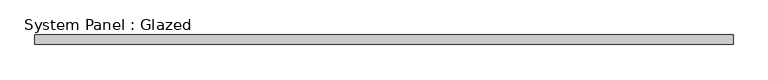
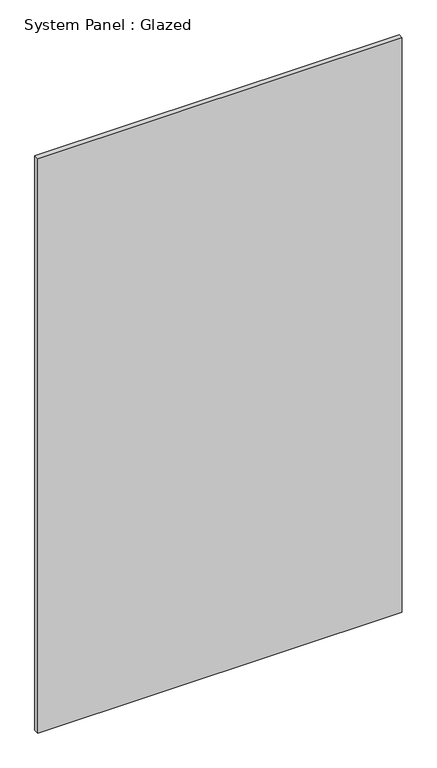
"""IFC4 building model written with IfcOpenShell, lengths in millimetres: plate geometry, System Panel : Glazed."""

from ifc_helpers import new_model, si_unit, origin, origin_with_axes, place, context, project, spatial, polyline, outline, extrude, source, transform, mapped, element, save


def system_panel_glazed_6661c6ea(model_context):
    return source(origin(), model_context, "Body", "SweptSolid", [
        extrude(outline(polyline([(915.0000002, 24.5), (-915.0000002, 24.5), (-915.0000002, 49.5), (915.0000002, 49.5), (915.0000002, 24.5)])), origin_with_axes(), (0.0, 0.0, 1.0), 3048.0),
    ])


if __name__ == "__main__":
    model = new_model("IFC4")
    model_context = context("Model", 3, world=origin())
    ifc_project = project(units=[si_unit("LENGTHUNIT", "METRE", prefix="MILLI")], contexts=[model_context])
    site = spatial("IfcSite", under=ifc_project)
    building = spatial("IfcBuilding", under=site)
    placement = place(None, origin())
    system_panel_glazed_shape = system_panel_glazed_6661c6ea(model_context)
    element("IfcPlate", 1, ObjectType="System Panel : Glazed", at=placement, inside=building, context=model_context, shape_type="MappedRepresentation", body=[
        mapped(system_panel_glazed_shape, transform((0.0, 0.0, 0.0), x_axis=(1.0, 0.0, 0.0), y_axis=(0.0, 1.0, 0.0), z_axis=(0.0, 0.0, 1.0))),
    ])
    save(model, "model.ifc")

# Revit data of these elements
# Type "System Panel : Glazed"
#   Keynote = "H11"
#   Construction Type Id = "GSP4R"
#   Analytic Construction = "1/8 in Pilkington single glazing"
#   Visual Light Transmittance = 0.9
#   Solar Heat Gain Coefficient = 0.86
#   Heat Transfer Coefficient (U) = 6.7069 W/(m²·K)
#   Define Thermal Properties by = 1
# Element 1 (IfcPlate, "System Panel : Glazed")
#   Materials on its faces: "Glass"
# Materials
#   "Glass": class "Glass", colour RGB 0 128 192, transparency 0.9, Description = "Soda Lime Glass", Cost = 0
